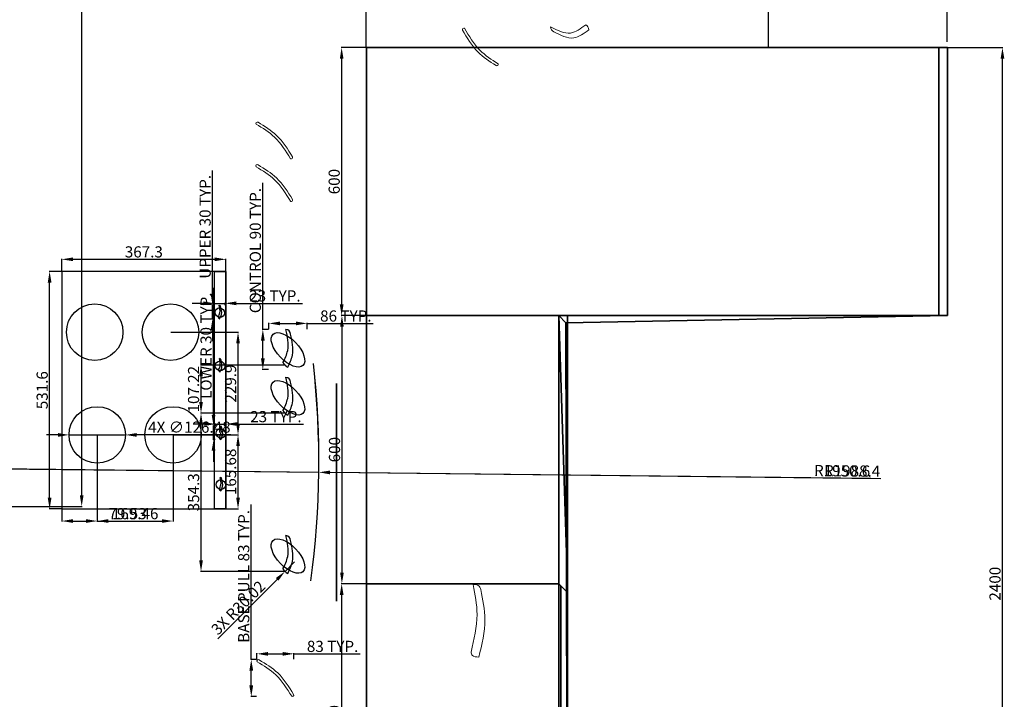
# Model space of a CAD drawing. Units: millimetres. Extents: x 11557 to 15272, y 8572 to 13242.
# Tile 3 of 4: x 13069 to 15272, y 9640 to 11161. Entities that reach past the tile are written whole.
import ezdxf

# ---------------------------------------------------------------- set-up
doc = ezdxf.new("R2010")
doc.units = ezdxf.units.MM
for name, color, linetype, lineweight in [('A-ANNO-DIMS', 2, 'Continuous', 18), ('A-ANNO-REFP', 8, 'Continuous', 13), ('A-EQPM', 9, 'Continuous', 25), ('A-FURN-BASE', 7, 'Continuous', 35), ('A-FURN-HARD', 8, 'Continuous', 18)]:
    doc.layers.add(name, color=color, linetype=linetype, lineweight=lineweight)
doc.styles.get("Standard").update_dxf_attribs({"font": 'arial.ttf'})
doc.dimstyles.new('ISO-25', dxfattribs={"dimtxt": 25, "dimasz": 25, "dimexe": 1.25, "dimexo": 0.625, "dimtad": 1, "dimdec": 1, "dimtxsty": 'Standard', "dimcen": 2.5, "dimadec": 0, "dimazin": 0, "dimtfac": 1, "dimtdec": 1, "dimtmove": 0, "dimatfit": 3, "dimfxl": 1, "dimarcsym": 0})

# ---------------------------------------------------------------- blocks, each defined once
blk = doc.blocks.new('*D2')
at = {"layer": 'A-ANNO-DIMS', "color": 0, "lineweight": -2, "transparency": 16777216}
for p, q in [((13844.6, 9898.9), (13788.4, 9898.9)), ((13789.6, 9873.9), (13789.6, 9323.9)), ((13844.6, 9298.9), (13788.4, 9298.9))]:
    blk.add_line(p, q, dxfattribs=at)
at = {"layer": 'A-ANNO-DIMS', "color": 0, "transparency": 16777216}
for points in [[(13785.5, 9873.9), (13793.8, 9873.9), (13789.6, 9898.9)], [(13785.5, 9323.9), (13793.8, 9323.9), (13789.6, 9298.9)]]:
    blk.add_solid(points, dxfattribs=at)
at = {"layer": 'Defpoints', "color": 0, "transparency": 16777216}
for p in [(13845.2, 9898.9, 720), (13789.6, 9298.9), (13845.2, 9298.9, 720)]:
    blk.add_point(p, dxfattribs=at)
at = {"layer": 'A-ANNO-DIMS', "color": 0, "transparency": 16777216, "insert": (13776.2, 9598.9), "char_height": 25, "attachment_point": 5, "rotation": 90}
blk.add_mtext('600', dxfattribs=at)
blk = doc.blocks.new('*D3')
at = {"layer": 'A-ANNO-DIMS', "color": 0, "lineweight": -2, "transparency": 16777216}
for p, q in [((13845.2, 10498.9), (13789, 10498.9)), ((13790.2, 10473.9), (13790.2, 9923.9)), ((13845.2, 9898.9), (13789, 9898.9))]:
    blk.add_line(p, q, dxfattribs=at)
at = {"layer": 'A-ANNO-DIMS', "color": 0, "transparency": 16777216}
for points in [[(13786.1, 10473.9), (13794.4, 10473.9), (13790.2, 10498.9)], [(13786.1, 9923.9), (13794.4, 9923.9), (13790.2, 9898.9)]]:
    blk.add_solid(points, dxfattribs=at)
at = {"layer": 'Defpoints', "color": 0, "transparency": 16777216}
for p in [(13845.9, 10498.9, 720), (13790.2, 9898.9), (13845.9, 9898.9, 720)]:
    blk.add_point(p, dxfattribs=at)
at = {"layer": 'A-ANNO-DIMS', "color": 0, "transparency": 16777216, "insert": (13776.9, 10198.9), "char_height": 25, "attachment_point": 5, "rotation": 90}
blk.add_mtext('600', dxfattribs=at)
blk = doc.blocks.new('*D4')
at = {"layer": 'A-ANNO-DIMS', "color": 0, "lineweight": -2, "transparency": 16777216}
for p, q in [((13844.6, 11098.9), (13788.4, 11098.9)), ((13789.6, 11073.9), (13789.6, 10523.9)), ((13844.6, 10498.9), (13788.4, 10498.9))]:
    blk.add_line(p, q, dxfattribs=at)
at = {"layer": 'A-ANNO-DIMS', "color": 0, "transparency": 16777216}
for points in [[(13785.5, 11073.9), (13793.8, 11073.9), (13789.6, 11098.9)], [(13785.5, 10523.9), (13793.8, 10523.9), (13789.6, 10498.9)]]:
    blk.add_solid(points, dxfattribs=at)
at = {"layer": 'Defpoints', "color": 0, "transparency": 16777216}
for p in [(13845.2, 11098.9, 720), (13789.6, 10498.9), (13845.2, 10498.9, 720)]:
    blk.add_point(p, dxfattribs=at)
at = {"layer": 'A-ANNO-DIMS', "color": 0, "transparency": 16777216, "insert": (13776.2, 10798.9), "char_height": 25, "attachment_point": 5, "rotation": 90}
blk.add_mtext('600', dxfattribs=at)
blk = doc.blocks.new('*D5')
at = {"layer": 'A-ANNO-DIMS', "color": 0, "lineweight": -2, "transparency": 16777216}
for p, q in [((13844.6, 11098.9), (13844.6, 11236.3)), ((13869.6, 11235), (14719.6, 11235)), ((14744.6, 11098.9), (14744.6, 11236.3))]:
    blk.add_line(p, q, dxfattribs=at)
at = {"layer": 'A-ANNO-DIMS', "color": 0, "transparency": 16777216}
for points in [[(13869.6, 11239.2), (13869.6, 11230.9), (13844.6, 11235)], [(14719.6, 11239.2), (14719.6, 11230.9), (14744.6, 11235)]]:
    blk.add_solid(points, dxfattribs=at)
at = {"layer": 'Defpoints', "color": 0, "transparency": 16777216}
for p in [(14744.6, 11235), (13844.6, 11098.2, 720), (14744.6, 11098.2, 720)]:
    blk.add_point(p, dxfattribs=at)
at = {"layer": 'A-ANNO-DIMS', "color": 0, "transparency": 16777216, "insert": (14294.6, 11248.4), "char_height": 25, "attachment_point": 5}
blk.add_mtext('900', dxfattribs=at)
blk = doc.blocks.new('*D6')
at = {"layer": 'A-ANNO-DIMS', "color": 0, "lineweight": -2, "transparency": 16777216}
for p, q in [((14744.6, 11111.7), (14744.6, 11236.3)), ((15119.6, 11235), (14769.6, 11235)), ((15144.6, 11111.7), (15144.6, 11236.3))]:
    blk.add_line(p, q, dxfattribs=at)
at = {"layer": 'A-ANNO-DIMS', "color": 0, "transparency": 16777216}
for points in [[(14769.6, 11239.2), (14769.6, 11230.9), (14744.6, 11235)], [(15119.6, 11239.2), (15119.6, 11230.9), (15144.6, 11235)]]:
    blk.add_solid(points, dxfattribs=at)
at = {"layer": 'Defpoints', "color": 0, "transparency": 16777216}
for p in [(14744.6, 11235), (14744.6, 11111, 720), (15144.6, 11111, 720)]:
    blk.add_point(p, dxfattribs=at)
at = {"layer": 'A-ANNO-DIMS', "color": 0, "transparency": 16777216, "insert": (14944.6, 11248.4), "char_height": 25, "attachment_point": 5}
blk.add_mtext('400', dxfattribs=at)
blk = doc.blocks.new('BASE-CABINET-PULL')
for centre, radius, start, end in [((3, 79.7, -122.8), 3.04, 50.0455, 215.1607), ((79.2, 3.1, -122.8), 3.13, 238.0113, 27.1949)]:
    blk.add_arc(centre, radius, start, end)
for points in [[(77.6, 0.5, -122.8), (66.9, 17.8, -122.8), (47.2, 49.7, -122.8), (15.2, 69.1, -122.8), (0.5, 77.9, -122.8)], [(82, 4.6, -122.8), (71.3, 21.8, -122.8), (51.6, 53.8, -122.8), (19.6, 73.1, -122.8), (5, 82, -122.8)]]:
    blk.add_open_spline(points, degree=3, knots=[0, 0, 0, 0, 59.935873, 110.632609, 110.632609, 110.632609, 110.632609])
blk = doc.blocks.new('HOB-BURNER')
for centre in [(63.2, 63.2), (63.2, 63.2, -14.7)]:
    blk.add_circle(centre, 63.2)
blk = doc.blocks.new('OVEN-CONTROL')
for centre, radius, start, end in [((31.7, 73), 11.8, 5.8892, 84.1108), ((52.1, 25.8), 30, 210.6614, 239.3386)]:
    blk.add_arc(centre, radius, start, end)
blk.add_ellipse((37.5, 39, 2.5), major_axis=(-33.5, 35), ratio=0.486746)
for points in [[(26.2, 10.5), (30.6, 19.4), (42, 42.9), (36.4, 68.7), (32.9, 84.8)], [(36.8, 0), (41.1, 8.9), (52.5, 32.3), (46.9, 58.2), (43.4, 74.2)]]:
    blk.add_open_spline(points, degree=3, knots=[0, 0, 0, 0, 29.141787, 76.393896, 76.393896, 76.393896, 76.393896])
blk = doc.blocks.new('HOB-CONTROL-LOWER')
for centre, radius, start, end in [((9, 25.8), 4.17, 5.8892, 84.1108), ((16.2, 9.1), 10.6, 210.6614, 239.3386)]:
    blk.add_arc(centre, radius, start, end)
blk.add_ellipse((10.6, 13.6, 1.1), major_axis=(-7.62, 7.96), ratio=0.928231)
for points in [[(7, 3.7), (8.6, 6.9), (12.6, 15.1), (10.6, 24.3), (9.4, 30)], [(10.7, 0), (12.3, 3.2), (16.3, 11.4), (14.3, 20.6), (13.1, 26.2)]]:
    blk.add_open_spline(points, degree=3, knots=[0, 0, 0, 0, 10.30237, 27.007204, 27.007204, 27.007204, 27.007204])
blk = doc.blocks.new('HOB-CONTROL-UPPER')
for centre, radius, start, end in [((9, 25.8, -1.1), 4.17, 5.8892, 84.1108), ((16.2, 9.1, -1.1), 10.6, 210.6614, 239.3386)]:
    blk.add_arc(centre, radius, start, end)
blk.add_ellipse((10.6, 13.6), major_axis=(-7.62, 7.96), ratio=0.928231)
for points in [[(7, 3.7, -1.1), (8.6, 6.9, -1.1), (12.6, 15.1, -1.1), (10.6, 24.3, -1.1), (9.4, 30, -1.1)], [(10.7, 0, -1.1), (12.3, 3.2, -1.1), (16.3, 11.4, -1.1), (14.3, 20.6, -1.1), (13.1, 26.2, -1.1)]]:
    blk.add_open_spline(points, degree=3, knots=[0, 0, 0, 0, 10.30237, 27.007204, 27.007204, 27.007204, 27.007204])
blk = doc.blocks.new('*D21')
at = {"layer": 'A-ANNO-DIMS', "color": 0, "lineweight": -2, "transparency": 16777216}
for p, q in [((13587.4, 9729.4), (13587.4, 10076.2)), ((13599.3, 9729.4), (13586.1, 9729.4)), ((13587.4, 9671.1), (13587.4, 9704.4)), ((13599.3, 9646.1), (13586.1, 9646.1))]:
    blk.add_line(p, q, dxfattribs=at)
at = {"layer": 'A-ANNO-DIMS', "color": 0, "transparency": 16777216}
for points in [[(13583.2, 9704.4), (13591.6, 9704.4), (13587.4, 9729.4)], [(13583.2, 9671.1), (13591.6, 9671.1), (13587.4, 9646.1)]]:
    blk.add_solid(points, dxfattribs=at)
at = {"layer": 'Defpoints', "color": 0, "transparency": 16777216}
for p in [(13587.4, 9729.4), (13599.9, 9729.4), (13599.9, 9646.1)]:
    blk.add_point(p, dxfattribs=at)
at = {"layer": 'A-ANNO-DIMS', "color": 0, "transparency": 16777216, "insert": (13573.8, 9915.3), "char_height": 25, "attachment_point": 5, "rotation": 90}
blk.add_mtext('BASE PULL 83 TYP.', dxfattribs=at)
blk = doc.blocks.new('*D22')
at = {"layer": 'A-ANNO-DIMS', "color": 0, "lineweight": -2, "transparency": 16777216}
for p, q in [((13599.9, 9730), (13599.9, 9743.1)), ((13624.9, 9741.9), (13657.9, 9741.9)), ((13682.9, 9730), (13682.9, 9743.1)), ((13682.9, 9741.9), (13830.8, 9741.9))]:
    blk.add_line(p, q, dxfattribs=at)
at = {"layer": 'A-ANNO-DIMS', "color": 0, "transparency": 16777216}
for points in [[(13624.9, 9746), (13624.9, 9737.7), (13599.9, 9741.9)], [(13657.9, 9746), (13657.9, 9737.7), (13682.9, 9741.9)]]:
    blk.add_solid(points, dxfattribs=at)
at = {"layer": 'Defpoints', "color": 0, "transparency": 16777216}
for p in [(13682.9, 9741.9), (13599.9, 9729.4), (13682.9, 9729.4)]:
    blk.add_point(p, dxfattribs=at)
at = {"layer": 'A-ANNO-DIMS', "color": 0, "transparency": 16777216, "insert": (13769.4, 9755.3), "char_height": 25, "attachment_point": 5}
blk.add_mtext('83 TYP.', dxfattribs=at)
blk = doc.blocks.new('*D23')
at = {"layer": 'A-ANNO-DIMS', "color": 0, "lineweight": -2, "transparency": 16777216}
for p, q in [((13613.3, 10468), (13613.3, 10796.1)), ((13626.1, 10468), (13612, 10468)), ((13613.3, 10403.2), (13613.3, 10443)), ((13626.1, 10378.2), (13612, 10378.2))]:
    blk.add_line(p, q, dxfattribs=at)
at = {"layer": 'A-ANNO-DIMS', "color": 0, "transparency": 16777216}
for points in [[(13609.1, 10443), (13617.5, 10443), (13613.3, 10468)], [(13609.1, 10403.2), (13617.5, 10403.2), (13613.3, 10378.2)]]:
    blk.add_solid(points, dxfattribs=at)
at = {"layer": 'Defpoints', "color": 0, "transparency": 16777216}
for p in [(13613.3, 10468), (13626.8, 10468), (13626.8, 10378.2)]:
    blk.add_point(p, dxfattribs=at)
at = {"layer": 'A-ANNO-DIMS', "color": 0, "transparency": 16777216, "insert": (13599.7, 10644.5), "char_height": 25, "attachment_point": 5, "rotation": 90}
blk.add_mtext('CONTROL 90 TYP.', dxfattribs=at)
blk = doc.blocks.new('*D24')
at = {"layer": 'A-ANNO-DIMS', "color": 0, "lineweight": -2, "transparency": 16777216}
for p, q in [((13626.8, 10468.6), (13626.8, 10482.7)), ((13651.8, 10481.4), (13687.5, 10481.4)), ((13712.5, 10468.6), (13712.5, 10482.7)), ((13712.5, 10481.4), (13860.5, 10481.4))]:
    blk.add_line(p, q, dxfattribs=at)
at = {"layer": 'A-ANNO-DIMS', "color": 0, "transparency": 16777216}
for points in [[(13651.8, 10485.6), (13651.8, 10477.3), (13626.8, 10481.4)], [(13687.5, 10485.6), (13687.5, 10477.3), (13712.5, 10481.4)]]:
    blk.add_solid(points, dxfattribs=at)
at = {"layer": 'Defpoints', "color": 0, "transparency": 16777216}
for p in [(13626.8, 10468), (13712.5, 10481.4), (13712.5, 10468)]:
    blk.add_point(p, dxfattribs=at)
at = {"layer": 'A-ANNO-DIMS', "color": 0, "transparency": 16777216, "insert": (13799, 10494.8), "char_height": 25, "attachment_point": 5}
blk.add_mtext('86 TYP.', dxfattribs=at)
blk = doc.blocks.new('*D29')
at = {"layer": 'A-ANNO-DIMS', "color": 0, "lineweight": -2, "transparency": 16777216}
for p, q in [((13503.1, 10276.7), (13503.1, 10561.3)), ((13506.9, 10251.7), (13501.8, 10251.7)), ((13503.1, 10221.7), (13503.1, 10251.7)), ((13506.9, 10221.7), (13501.8, 10221.7)), ((13503.1, 10196.7), (13503.1, 10171.7))]:
    blk.add_line(p, q, dxfattribs=at)
at = {"layer": 'A-ANNO-DIMS', "color": 0, "transparency": 16777216}
for points in [[(13498.9, 10276.7), (13507.2, 10276.7), (13503.1, 10251.7)], [(13498.9, 10196.7), (13507.2, 10196.7), (13503.1, 10221.7)]]:
    blk.add_solid(points, dxfattribs=at)
at = {"layer": 'Defpoints', "color": 0, "transparency": 16777216}
for p in [(13503.1, 10251.7), (13507.6, 10251.7), (13507.6, 10221.7)]:
    blk.add_point(p, dxfattribs=at)
at = {"layer": 'A-ANNO-DIMS', "color": 0, "transparency": 16777216, "insert": (13489.5, 10431.5), "char_height": 25, "attachment_point": 5, "rotation": 90}
blk.add_mtext('LOWER 30 TYP.', dxfattribs=at)
blk = doc.blocks.new('*D30')
at = {"layer": 'A-ANNO-DIMS', "color": 0, "lineweight": -2, "transparency": 16777216}
for p, q in [((13482.6, 10256.2), (13457.6, 10256.2)), ((13507.6, 10252.3), (13507.6, 10257.4)), ((13507.6, 10256.2), (13531, 10256.2)), ((13531, 10252.3), (13531, 10257.4)), ((13556, 10256.2), (13704.3, 10256.2))]:
    blk.add_line(p, q, dxfattribs=at)
at = {"layer": 'A-ANNO-DIMS', "color": 0, "transparency": 16777216}
for points in [[(13482.6, 10260.4), (13482.6, 10252), (13507.6, 10256.2)], [(13556, 10260.4), (13556, 10252), (13531, 10256.2)]]:
    blk.add_solid(points, dxfattribs=at)
at = {"layer": 'Defpoints', "color": 0, "transparency": 16777216}
for p in [(13507.6, 10251.7), (13531, 10256.2), (13531, 10251.7)]:
    blk.add_point(p, dxfattribs=at)
at = {"layer": 'A-ANNO-DIMS', "color": 0, "transparency": 16777216, "insert": (13642.6, 10269.6), "char_height": 25, "attachment_point": 5}
blk.add_mtext('23 TYP.', dxfattribs=at)
blk = doc.blocks.new('*D31')
at = {"layer": 'A-ANNO-DIMS', "color": 0, "lineweight": -2, "transparency": 16777216}
for p, q in [((13500.8, 10546.9), (13500.8, 10823.6)), ((13504.6, 10521.9), (13499.5, 10521.9)), ((13500.8, 10491.9), (13500.8, 10521.9)), ((13504.6, 10491.9), (13499.5, 10491.9)), ((13500.8, 10466.9), (13500.8, 10441.9))]:
    blk.add_line(p, q, dxfattribs=at)
at = {"layer": 'A-ANNO-DIMS', "color": 0, "transparency": 16777216}
for points in [[(13496.6, 10546.9), (13504.9, 10546.9), (13500.8, 10521.9)], [(13496.6, 10466.9), (13504.9, 10466.9), (13500.8, 10491.9)]]:
    blk.add_solid(points, dxfattribs=at)
at = {"layer": 'Defpoints', "color": 0, "transparency": 16777216}
for p in [(13500.8, 10521.9), (13505.3, 10521.9), (13505.3, 10491.9)]:
    blk.add_point(p, dxfattribs=at)
at = {"layer": 'A-ANNO-DIMS', "color": 0, "transparency": 16777216, "insert": (13487.4, 10697.7), "char_height": 25, "attachment_point": 5, "rotation": 90}
blk.add_mtext('UPPER 30 TYP.', dxfattribs=at)
blk = doc.blocks.new('*D32')
at = {"layer": 'A-ANNO-DIMS', "color": 0, "lineweight": -2, "transparency": 16777216}
for p, q in [((13480.3, 10526.4), (13455.3, 10526.4)), ((13505.3, 10522.5), (13505.3, 10527.6)), ((13505.3, 10526.4), (13528.7, 10526.4)), ((13528.7, 10522.5), (13528.7, 10527.6)), ((13553.7, 10526.4), (13702, 10526.4))]:
    blk.add_line(p, q, dxfattribs=at)
at = {"layer": 'A-ANNO-DIMS', "color": 0, "transparency": 16777216}
for points in [[(13480.3, 10530.6), (13480.3, 10522.2), (13505.3, 10526.4)], [(13553.7, 10530.6), (13553.7, 10522.2), (13528.7, 10526.4)]]:
    blk.add_solid(points, dxfattribs=at)
at = {"layer": 'Defpoints', "color": 0, "transparency": 16777216}
for p in [(13505.3, 10521.9), (13528.7, 10526.4), (13528.7, 10521.9)]:
    blk.add_point(p, dxfattribs=at)
at = {"layer": 'A-ANNO-DIMS', "color": 0, "transparency": 16777216, "insert": (13640.3, 10539.8), "char_height": 25, "attachment_point": 5}
blk.add_mtext('23 TYP.', dxfattribs=at)
blk = doc.blocks.new('*D35')
at = {"layer": 'A-ANNO-DIMS', "color": 0, "lineweight": -2, "transparency": 16777216}
for p, q in [((15145.9, 11098.9), (15269.1, 11098.9)), ((15267.9, 8723.9), (15267.9, 11073.9)), ((14295.9, 8698.9), (15269.1, 8698.9))]:
    blk.add_line(p, q, dxfattribs=at)
at = {"layer": 'A-ANNO-DIMS', "color": 0, "transparency": 16777216}
for points in [[(15263.7, 11073.9), (15272.1, 11073.9), (15267.9, 11098.9)], [(15263.7, 8723.9), (15272.1, 8723.9), (15267.9, 8698.9)]]:
    blk.add_solid(points, dxfattribs=at)
at = {"layer": 'Defpoints', "color": 0, "transparency": 16777216}
for p in [(15145.2, 11098.9), (15267.9, 11098.9), (14295.2, 8698.9)]:
    blk.add_point(p, dxfattribs=at)
at = {"layer": 'A-ANNO-DIMS', "color": 0, "transparency": 16777216, "insert": (15254.5, 9898.9), "char_height": 25, "attachment_point": 5, "rotation": 90}
blk.add_mtext('2400', dxfattribs=at)
blk = doc.blocks.new('*D36')
at = {"layer": 'A-ANNO-DIMS', "color": 0, "lineweight": -2, "transparency": 16777216}
for p, q in [((12944.4, 13071.7), (13209.3, 13071.7)), ((13208.1, 10096.7), (13208.1, 13046.7)), ((11895, 10071.7), (13209.3, 10071.7))]:
    blk.add_line(p, q, dxfattribs=at)
at = {"layer": 'A-ANNO-DIMS', "color": 0, "transparency": 16777216}
for points in [[(13203.9, 13046.7), (13212.2, 13046.7), (13208.1, 13071.7)], [(13203.9, 10096.7), (13212.2, 10096.7), (13208.1, 10071.7)]]:
    blk.add_solid(points, dxfattribs=at)
at = {"layer": 'Defpoints', "color": 0, "transparency": 16777216}
for p in [(12943.8, 13071.7), (13208.1, 13071.7), (11894.4, 10071.7)]:
    blk.add_point(p, dxfattribs=at)
at = {"layer": 'A-ANNO-DIMS', "color": 0, "transparency": 16777216, "insert": (13194.7, 11571.7), "char_height": 25, "attachment_point": 5, "rotation": 90}
blk.add_mtext('3000', dxfattribs=at)
blk = doc.blocks.new('*D41')
at = {"layer": 'A-ANNO-DIMS', "color": 0, "lineweight": -2, "transparency": 16777216}
for p, q in [((13163.4, 10598.5), (13163.4, 10626.2)), ((13188.4, 10624.9), (13505.7, 10624.9)), ((13530.7, 10598.5), (13530.7, 10626.2))]:
    blk.add_line(p, q, dxfattribs=at)
at = {"layer": 'A-ANNO-DIMS', "color": 0, "transparency": 16777216}
for points in [[(13188.4, 10629.1), (13188.4, 10620.8), (13163.4, 10624.9)], [(13505.7, 10629.1), (13505.7, 10620.8), (13530.7, 10624.9)]]:
    blk.add_solid(points, dxfattribs=at)
at = {"layer": 'Defpoints', "color": 0, "transparency": 16777216}
for p in [(13530.7, 10624.9), (13163.4, 10597.8), (13530.7, 10597.8)]:
    blk.add_point(p, dxfattribs=at)
at = {"layer": 'A-ANNO-DIMS', "color": 0, "transparency": 16777216, "insert": (13347.1, 10638.3), "char_height": 25, "attachment_point": 5}
blk.add_mtext('367.3', dxfattribs=at)
blk = doc.blocks.new('*D42')
at = {"layer": 'A-ANNO-DIMS', "color": 0, "lineweight": -2, "transparency": 16777216}
for p, q in [((13162.8, 10597.8), (13135.1, 10597.8)), ((13136.3, 10091.2), (13136.3, 10572.8)), ((13162.8, 10066.2), (13135.1, 10066.2))]:
    blk.add_line(p, q, dxfattribs=at)
at = {"layer": 'A-ANNO-DIMS', "color": 0, "transparency": 16777216}
for points in [[(13132.1, 10572.8), (13140.5, 10572.8), (13136.3, 10597.8)], [(13132.1, 10091.2), (13140.5, 10091.2), (13136.3, 10066.2)]]:
    blk.add_solid(points, dxfattribs=at)
at = {"layer": 'Defpoints', "color": 0, "transparency": 16777216}
for p in [(13136.3, 10597.8), (13163.4, 10597.8), (13163.4, 10066.2)]:
    blk.add_point(p, dxfattribs=at)
at = {"layer": 'A-ANNO-DIMS', "color": 0, "transparency": 16777216, "insert": (13122.9, 10332), "char_height": 25, "attachment_point": 5, "rotation": 90}
blk.add_mtext('531.6', dxfattribs=at)
blk = doc.blocks.new('*D43')
at = {"layer": 'A-ANNO-DIMS', "color": 0, "lineweight": -2, "transparency": 16777216}
for p, q in [((13242.9, 10231.3), (13242.9, 10037.9)), ((13412.4, 10231.3), (13412.4, 10037.9)), ((13267.9, 10039.1), (13387.4, 10039.1))]:
    blk.add_line(p, q, dxfattribs=at)
at = {"layer": 'A-ANNO-DIMS', "color": 0, "transparency": 16777216}
for points in [[(13267.9, 10043.3), (13267.9, 10035), (13242.9, 10039.1)], [(13387.4, 10043.3), (13387.4, 10035), (13412.4, 10039.1)]]:
    blk.add_solid(points, dxfattribs=at)
at = {"layer": 'Defpoints', "color": 0, "transparency": 16777216}
for p in [(13242.9, 10231.9), (13412.4, 10231.9), (13412.4, 10039.1)]:
    blk.add_point(p, dxfattribs=at)
at = {"layer": 'A-ANNO-DIMS', "color": 0, "transparency": 16777216, "insert": (13327.7, 10052.5), "char_height": 25, "attachment_point": 5}
blk.add_mtext('169.46', dxfattribs=at)
blk = doc.blocks.new('*D44')
at = {"layer": 'A-ANNO-DIMS', "color": 0, "lineweight": -2, "transparency": 16777216}
for p, q in [((13407.3, 10461.8), (13559.1, 10461.8)), ((13557.8, 10256.9), (13557.8, 10436.8)), ((13413, 10231.9), (13559.1, 10231.9))]:
    blk.add_line(p, q, dxfattribs=at)
at = {"layer": 'A-ANNO-DIMS', "color": 0, "transparency": 16777216}
for points in [[(13553.7, 10436.8), (13562, 10436.8), (13557.8, 10461.8)], [(13553.7, 10256.9), (13562, 10256.9), (13557.8, 10231.9)]]:
    blk.add_solid(points, dxfattribs=at)
at = {"layer": 'Defpoints', "color": 0, "transparency": 16777216}
for p in [(13406.6, 10461.8), (13557.8, 10461.8), (13412.4, 10231.9)]:
    blk.add_point(p, dxfattribs=at)
at = {"layer": 'A-ANNO-DIMS', "color": 0, "transparency": 16777216, "insert": (13544.4, 10346.8), "char_height": 25, "attachment_point": 5, "rotation": 90}
blk.add_mtext('229.9', dxfattribs=at)
blk = doc.blocks.new('*D45')
at = {"layer": 'A-ANNO-DIMS', "color": 0, "lineweight": -2, "transparency": 16777216}
for p, q in [((13242.9, 10231.3), (13242.9, 10037.9)), ((13163.4, 10065.6), (13163.4, 10037.9)), ((13188.4, 10039.1), (13217.9, 10039.1)), ((13242.9, 10039.1), (13353.4, 10039.1))]:
    blk.add_line(p, q, dxfattribs=at)
at = {"layer": 'A-ANNO-DIMS', "color": 0, "transparency": 16777216}
for points in [[(13188.4, 10043.3), (13188.4, 10035), (13163.4, 10039.1)], [(13217.9, 10043.3), (13217.9, 10035), (13242.9, 10039.1)]]:
    blk.add_solid(points, dxfattribs=at)
at = {"layer": 'Defpoints', "color": 0, "transparency": 16777216}
for p in [(13242.9, 10231.9), (13163.4, 10066.2), (13242.9, 10039.1)]:
    blk.add_point(p, dxfattribs=at)
at = {"layer": 'A-ANNO-DIMS', "color": 0, "transparency": 16777216, "insert": (13310.6, 10052.5), "char_height": 25, "attachment_point": 5}
blk.add_mtext('79.53', dxfattribs=at)
blk = doc.blocks.new('*D46')
at = {"layer": 'A-ANNO-DIMS', "color": 0, "lineweight": -2, "transparency": 16777216}
for p, q in [((13413, 10231.9), (13559.1, 10231.9)), ((13557.8, 10091.2), (13557.8, 10206.9)), ((13531.4, 10066.2), (13559.1, 10066.2))]:
    blk.add_line(p, q, dxfattribs=at)
at = {"layer": 'A-ANNO-DIMS', "color": 0, "transparency": 16777216}
for points in [[(13553.7, 10206.9), (13562, 10206.9), (13557.8, 10231.9)], [(13553.7, 10091.2), (13562, 10091.2), (13557.8, 10066.2)]]:
    blk.add_solid(points, dxfattribs=at)
at = {"layer": 'Defpoints', "color": 0, "transparency": 16777216}
for p in [(13412.4, 10231.9), (13557.8, 10231.9), (13530.7, 10066.2)]:
    blk.add_point(p, dxfattribs=at)
at = {"layer": 'A-ANNO-DIMS', "color": 0, "transparency": 16777216, "insert": (13544.4, 10149.1), "char_height": 25, "attachment_point": 5, "rotation": 90}
blk.add_mtext('165.68', dxfattribs=at)
blk = doc.blocks.new('*D47')
at = {"layer": 'A-ANNO-DIMS', "color": 0, "lineweight": -2, "transparency": 16777216}
for p, q in [((13662.3, 10280.6), (13473.8, 10280.6)), ((13475, 9951.3), (13475, 10255.6)), ((13662.3, 9926.3), (13473.8, 9926.3))]:
    blk.add_line(p, q, dxfattribs=at)
at = {"layer": 'A-ANNO-DIMS', "color": 0, "transparency": 16777216}
for points in [[(13470.8, 10255.6), (13479.2, 10255.6), (13475, 10280.6)], [(13470.8, 9951.3), (13479.2, 9951.3), (13475, 9926.3)]]:
    blk.add_solid(points, dxfattribs=at)
at = {"layer": 'Defpoints', "color": 0, "transparency": 16777216}
for p in [(13475, 10280.6), (13662.9, 10280.6), (13662.9, 9926.3)]:
    blk.add_point(p, dxfattribs=at)
at = {"layer": 'A-ANNO-DIMS', "color": 0, "transparency": 16777216, "insert": (13461.6, 10103.5), "char_height": 25, "attachment_point": 5, "rotation": 90}
blk.add_mtext('354.3', dxfattribs=at)
blk = doc.blocks.new('*D48')
at = {"layer": 'A-ANNO-DIMS', "color": 0, "lineweight": -2, "transparency": 16777216}
for p, q in [((13662.3, 10387.8), (13473.8, 10387.8)), ((13475, 10305.6), (13475, 10362.8)), ((13662.3, 10280.6), (13473.8, 10280.6))]:
    blk.add_line(p, q, dxfattribs=at)
at = {"layer": 'A-ANNO-DIMS', "color": 0, "transparency": 16777216}
for points in [[(13470.8, 10362.8), (13479.2, 10362.8), (13475, 10387.8)], [(13470.8, 10305.6), (13479.2, 10305.6), (13475, 10280.6)]]:
    blk.add_solid(points, dxfattribs=at)
at = {"layer": 'Defpoints', "color": 0, "transparency": 16777216}
for p in [(13475, 10387.8), (13662.9, 10387.8), (13662.9, 10280.6)]:
    blk.add_point(p, dxfattribs=at)
at = {"layer": 'A-ANNO-DIMS', "color": 0, "transparency": 16777216, "insert": (13461.6, 10334.2), "char_height": 25, "attachment_point": 5, "rotation": 90}
blk.add_mtext('107.22', dxfattribs=at)
blk = doc.blocks.new('*D50')
at = {"layer": 'A-ANNO-DIMS', "color": 0, "lineweight": -2, "transparency": 16777216}
for p, q in [((13154.7, 10231.9), (13129.7, 10231.9)), ((13179.7, 10231.9), (13306.2, 10231.9)), ((13541.9, 10231.9), (13331.2, 10231.9))]:
    blk.add_line(p, q, dxfattribs=at)
at = {"layer": 'A-ANNO-DIMS', "color": 0, "transparency": 16777216}
for points in [[(13154.7, 10236.1), (13154.7, 10227.7), (13179.7, 10231.9)], [(13331.2, 10236.1), (13331.2, 10227.7), (13306.2, 10231.9)]]:
    blk.add_solid(points, dxfattribs=at)
at = {"layer": 'Defpoints', "color": 0, "transparency": 16777216}
for p in [(13179.7, 10231.9), (13306.2, 10231.9)]:
    blk.add_point(p, dxfattribs=at)
at = {"layer": 'A-ANNO-DIMS', "color": 0, "transparency": 16777216, "insert": (13449, 10246), "char_height": 25, "attachment_point": 5, "rotation": 359.9999}
blk.add_mtext('4X ∅126.48', dxfattribs=at)
blk = doc.blocks.new('*D51')
at = {"layer": 'A-ANNO-DIMS', "color": 0, "lineweight": -2, "transparency": 16777216}
for p, q in [((13684.2, 9947.5), (13662.9, 9926.3)), ((13512.3, 9775.7), (13645.2, 9908.6))]:
    blk.add_line(p, q, dxfattribs=at)
at = {"layer": 'A-ANNO-DIMS', "color": 0, "transparency": 16777216}
blk.add_solid([(13642.3, 9911.6), (13648.2, 9905.7), (13662.9, 9926.3)], dxfattribs=at)
at = {"layer": 'Defpoints', "color": 0, "transparency": 16777216}
for p in [(13684.2, 9947.5), (13662.9, 9926.3)]:
    blk.add_point(p, dxfattribs=at)
at = {"layer": 'A-ANNO-DIMS', "color": 0, "transparency": 16777216, "insert": (13560.5, 9842.8), "char_height": 25, "attachment_point": 5, "rotation": 45.0002}
blk.add_mtext('3X R30.02', dxfattribs=at)
blk = doc.blocks.new('*D52')
at = {"layer": 'A-ANNO-DIMS', "color": 0, "lineweight": -2, "transparency": 16777216}
for p, q in [((11750.2, 10170.7), (13738.5, 10148.2)), ((14995.9, 10133.9), (13763.5, 10147.9))]:
    blk.add_line(p, q, dxfattribs=at)
at = {"layer": 'A-ANNO-DIMS', "color": 0, "transparency": 16777216}
blk.add_solid([(13763.5, 10152), (13763.4, 10143.7), (13738.5, 10148.2)], dxfattribs=at)
at = {"layer": 'Defpoints', "color": 0, "transparency": 16777216}
for p in [(11750.2, 10170.7), (13738.5, 10148.2)]:
    blk.add_point(p, dxfattribs=at)
at = {"layer": 'A-ANNO-DIMS', "color": 0, "transparency": 16777216, "insert": (14931.6, 10148), "char_height": 25, "attachment_point": 5, "rotation": 359.3508}
blk.add_mtext('R1988.4', dxfattribs=at)
blk = doc.blocks.new('*D53')
at = {"layer": 'A-ANNO-DIMS', "color": 0, "lineweight": -2, "transparency": 16777216}
for p, q in [((11788.3, 10170.3), (13738.8, 10148.2)), ((14973.5, 10134.2), (13763.8, 10147.9))]:
    blk.add_line(p, q, dxfattribs=at)
at = {"layer": 'A-ANNO-DIMS', "color": 0, "transparency": 16777216}
blk.add_solid([(13763.8, 10152), (13763.7, 10143.7), (13738.8, 10148.2)], dxfattribs=at)
at = {"layer": 'Defpoints', "color": 0, "transparency": 16777216}
for p in [(11788.3, 10170.3), (13738.8, 10148.2)]:
    blk.add_point(p, dxfattribs=at)
at = {"layer": 'A-ANNO-DIMS', "color": 0, "transparency": 16777216, "insert": (14909.2, 10148.3), "char_height": 25, "attachment_point": 5, "rotation": 359.3508}
blk.add_mtext('R1950.6', dxfattribs=at)

msp = doc.modelspace()

# ---------------------------------------------------------------- linework, layer by layer
at = {"layer": 'A-ANNO-REFP'}
for p in [(14745.243, 10498.859, 569.986), (14745.243, 10498.859, 419.972), (14745.243, 10498.859, 269.958), (14295.243, 10198.859, 556.518), (14295.243, 10198.859, 393.037), (14295.243, 10198.859, 229.555)]:
    msp.add_point(p, dxfattribs=at)
at = {"layer": 'A-EQPM'}
for p, q in [((13726.305, 10391.552), (13726.305, 10391.552, -30.747)), ((13778.188, 9859.679), (13778.188, 10346.865)), ((13778.188, 10346.865), (13778.188, 10346.865, -218.015)), ((13778.188, 10346.865, -218.015), (13778.188, 9859.679, -218.015)), ((13720.793, 9905.114), (13720.793, 9905.114, -30.747)), ((13778.188, 9859.679, -218.015), (13778.188, 9859.679))]:
    msp.add_line(p, q, dxfattribs=at)
for points in [[(13163.411, 10066.22), (13530.737, 10066.22), (13530.737, 10597.831), (13163.411, 10597.831)], [(13530.737, 10066.22), (13504.841, 10066.22), (13504.841, 10597.831), (13530.737, 10597.831)]]:
    msp.add_lwpolyline(points, close=True, dxfattribs=at)
for centre, radius, start, end in [((11788.258, 10170.261), 1950.639, 352.187696, 6.513961), ((11750.209, 10170.692, -30.747), 1988.4, 352.32442, 6.377237)]:
    msp.add_arc(centre, radius, start, end, dxfattribs=at)
at = {"layer": 'A-FURN-BASE'}
for p, q in [((13845.243, 10498.859, 720), (13845.243, 11098.859, 720)), ((13845.243, 11098.859, 720), (14745.243, 11098.859, 720)), ((14745.243, 11098.859, 720), (15145.243, 11098.859, 720)), ((15125.243, 10498.859, 720), (15125.243, 11098.859, 720)), ((15145.243, 11098.859, 720), (15145.243, 11098.859)), ((15145.243, 10498.859, 720), (15145.243, 11098.859, 720)), ((15145.243, 11098.859), (15145.243, 10498.859)), ((15145.243, 11098.859, 120), (15145.243, 10498.859, 120)), ((15145.243, 11098.859, 140), (15145.243, 10498.859, 140)), ((15145.243, 10528.859, 120), (15145.243, 10528.859)), ((15145.243, 10518.859, 120), (15145.243, 10518.859, 720)), ((15145.243, 10518.859, 120), (15145.243, 10518.859)), ((13845.243, 9898.859, 720), (13845.243, 10498.859, 720)), ((13845.243, 10498.859, 720), (14295.243, 10498.859, 720)), ((13845.243, 10498.859, 720), (14745.243, 10498.859, 720)), ((14275.243, 10498.859, 700), (14295.243, 9898.859, 720)), ((14275.243, 9298.859, 720), (14275.243, 10498.859, 720)), ((14275.243, 10498.859, 720), (14291.462, 10482.64, 136.098)), ((14275.243, 10498.859, 700), (14745.243, 10498.859, 700)), ((15145.243, 10498.859, 120), (14291.462, 10482.64, 136.098)), ((14745.243, 10498.859), (14295.243, 10498.859)), ((14295.243, 10478.859), (14295.243, 10498.859)), ((14295.243, 10498.859), (14295.243, 10498.859, 119.881)), ((14745.243, 10498.859, 720), (15145.243, 10498.859, 720)), ((14745.243, 10498.859, 720), (14745.243, 10498.859, 119.944)), ((14745.243, 10498.859, 569.986), (15145.243, 10498.859, 569.986)), ((14745.243, 10498.859, 419.972), (15145.243, 10498.859, 419.972)), ((14745.243, 10498.859, 269.958), (15145.243, 10498.859, 269.958)), ((15145.243, 10498.859), (14745.243, 10498.859)), ((14745.243, 10498.859, 700), (15145.243, 10498.859, 700)), ((15125.243, 10498.859, 720), (15125.243, 10498.859, 700)), ((15145.243, 10498.859, 120), (15145.243, 10498.859, 720)), ((14291.462, 10482.64, 136.098), (14295.243, 8708.859, 136.098)), ((14295.243, 9278.848), (14295.243, 10478.859)), ((14295.243, 10198.859, 720), (14292.06, 10202.042, 136.098)), ((13845.243, 9298.859, 720), (13845.243, 9898.859, 720)), ((13845.243, 9898.859, 720), (14275.243, 9898.859, 720)), ((14275.243, 9898.859, 720), (14292.744, 9881.358, 136.098)), ((14280.219, 9293.883, 565.291), (14280.219, 9893.883, 565.291)), ((14280.219, 9293.883, 237.922), (14280.219, 9893.883, 237.922)), ((14295.243, 9898.859, 720), (14295.243, 9298.859, 720))]:
    msp.add_line(p, q, dxfattribs=at)
at = {"layer": 'A-FURN-HARD'}
for centre, radius, start, end in [((14330.158, 11138.158), 12.644, 2.326481, 64.265858), ((14330.158, 11138.158, -152.015), 12.644, 2.326481, 64.265858), ((14330.158, 11138.158, -296.009), 12.644, 2.326481, 64.265858), ((14330.158, 11138.158, -441.162), 12.644, 2.326481, 64.265858), ((14062.814, 11139.559), 3.132, 56.524019, 205.70753), ((14269.434, 11145.621), 12.336, 181.465447, 245.126893), ((14269.434, 11145.621, -152.015), 12.336, 181.465447, 245.126893), ((14269.434, 11145.621, -296.009), 12.336, 181.465447, 245.126893), ((14269.434, 11145.621, -441.162), 12.336, 181.465447, 245.126893), ((14136.988, 11061.03), 3.045, 228.55821, 33.673339), ((14087.316, 9883.638), 13.754, 7.963069, 106.22766)]:
    msp.add_arc(centre, radius, start, end, dxfattribs=at)
for points, knots in [([(14257.102, 11145.305), (14272.249, 11137.422), (14299.915, 11123.024), (14324.516, 11141.284), (14335.648, 11149.547)], [0, 0, 0, 0, 46.62950242, 85.16957367, 85.16957367, 85.16957367, 85.16957367]), ([(14257.102, 11145.305, -152.015), (14272.249, 11137.422, -152.015), (14299.915, 11123.024, -152.015), (14324.516, 11141.284, -152.015), (14335.648, 11149.547, -152.015)], [0, 0, 0, 0, 46.62950242, 85.16957367, 85.16957367, 85.16957367, 85.16957367]), ([(14257.102, 11145.305, -296.009), (14272.249, 11137.422, -296.009), (14299.915, 11123.024, -296.009), (14324.516, 11141.284, -296.009), (14335.648, 11149.547, -296.009)], [0, 0, 0, 0, 46.62950242, 85.16957367, 85.16957367, 85.16957367, 85.16957367]), ([(14257.102, 11145.305, -441.162), (14272.249, 11137.422, -441.162), (14299.915, 11123.024, -441.162), (14324.516, 11141.284, -441.162), (14335.648, 11149.547, -441.162)], [0, 0, 0, 0, 46.62950242, 85.16957367, 85.16957367, 85.16957367, 85.16957367]), ([(14059.993, 11138.201), (14070.221, 11120.642), (14089.1, 11088.231), (14120.557, 11068.012), (14134.972, 11058.747)], [0, 0, 0, 0, 59.9358726, 110.63260885, 110.63260885, 110.63260885, 110.63260885]), ([(14064.542, 11142.172), (14074.77, 11124.613), (14093.649, 11092.202), (14125.106, 11071.983), (14139.521, 11062.718)], [0, 0, 0, 0, 59.9358726, 110.63260885, 110.63260885, 110.63260885, 110.63260885]), ([(14264.245, 11134.428), (14279.392, 11126.545), (14307.058, 11112.147), (14331.66, 11130.408), (14342.792, 11138.671)], [0, 0, 0, 0, 46.62950242, 85.16957367, 85.16957367, 85.16957367, 85.16957367]), ([(14264.245, 11134.428, -152.015), (14279.392, 11126.545, -152.015), (14307.058, 11112.147, -152.015), (14331.66, 11130.408, -152.015), (14342.792, 11138.671, -152.015)], [0, 0, 0, 0, 46.62950242, 85.16957367, 85.16957367, 85.16957367, 85.16957367]), ([(14264.245, 11134.428, -296.009), (14279.392, 11126.545, -296.009), (14307.058, 11112.147, -296.009), (14331.66, 11130.408, -296.009), (14342.792, 11138.671, -296.009)], [0, 0, 0, 0, 46.62950242, 85.16957367, 85.16957367, 85.16957367, 85.16957367]), ([(14264.245, 11134.428, -441.162), (14279.392, 11126.545, -441.162), (14307.058, 11112.147, -441.162), (14331.66, 11130.408, -441.162), (14342.792, 11138.671, -441.162)], [0, 0, 0, 0, 46.62950242, 85.16957367, 85.16957367, 85.16957367, 85.16957367]), ([(14079.013, 9745.963), (14085.864, 9773.97), (14098.135, 9824.132), (14087.965, 9874.568), (14083.473, 9896.844)], [0, 0, 0, 0, 85.19241077, 152.5838034, 152.5838034, 152.5838034, 152.5838034]), ([(14096.477, 9734.663), (14103.328, 9762.67), (14115.599, 9812.832), (14105.429, 9863.268), (14100.937, 9885.544)], [0, 0, 0, 0, 85.19241077, 152.5838034, 152.5838034, 152.5838034, 152.5838034]), ([(14079.013, 9745.963), (14079.754, 9743.059), (14081.817, 9734.975), (14090.752, 9734.785), (14096.477, 9734.663)], [0, 0, 0, 0, 8.29929483, 23.09865067, 23.09865067, 23.09865067, 23.09865067])]:
    msp.add_open_spline(points, degree=3, knots=knots, dxfattribs=at)

# ---------------------------------------------------------------- block references
at = {"layer": 'A-EQPM'}
for name, p in [('HOB-BURNER', (13173.941, 10398.555)), ('HOB-BURNER', (13343.404, 10398.555)), ('HOB-CONTROL-UPPER', (13506.349, 10491.943)), ('OVEN-CONTROL', (13632.082, 10383.229)), ('HOB-CONTROL-UPPER', (13506.928, 10372.633)), ('OVEN-CONTROL', (13632.082, 10276.008)), ('HOB-BURNER', (13179.703, 10168.66)), ('HOB-BURNER', (13349.166, 10168.66)), ('HOB-CONTROL-LOWER', (13508.648, 10221.734)), ('HOB-CONTROL-LOWER', (13508.648, 10106.78)), ('OVEN-CONTROL', (13632.082, 9921.718))]:
    msp.add_blockref(name, p, dxfattribs=at)
at = {"layer": 'A-FURN-HARD'}
for p in [(13597.647, 10849.545), (13597.647, 10754.239), (13600.211, 9646.362)]:
    msp.add_blockref('BASE-CABINET-PULL', p, dxfattribs=at)

# ---------------------------------------------------------------- dimensions: what is measured, and where the dimension line sits
at = {"layer": 'A-ANNO-DIMS'}
for base, p1, p2, override, picture, middle in [((13208.076, 13071.656), (11894.396, 10071.656), (12943.771, 13071.656), {"dimdec": 0, "dimlfac": 1, "dimrnd": 0, "dimzin": 0, "dimdsep": 46, "dimlunit": 2}, '*D36', (13194.678, 11571.656)), ((15267.893, 11098.859), (14295.243, 8698.859), (15145.243, 11098.859), {"dimdec": 0, "dimlfac": 1, "dimrnd": 0, "dimzin": 0, "dimdsep": 46, "dimlunit": 2}, '*D35', (15254.503, 9898.859)), ((13136.311, 10597.831), (13163.411, 10066.22), (13163.411, 10597.831), {"dimdec": 1, "dimlfac": 1, "dimrnd": 0, "dimzin": 0, "dimdsep": 46, "dimlunit": 2}, '*D42', (13122.913, 10332.026)), ((13557.837, 10461.797), (13412.407, 10231.902), (13406.646, 10461.797), {"dimdec": 1, "dimlfac": 1, "dimrnd": 0, "dimzin": 0, "dimdsep": 46, "dimlunit": 2}, '*D44', (13544.448, 10346.85)), ((13475.006, 10387.825), (13662.922, 10280.604), (13662.922, 10387.825), {"dimdec": 2, "dimlfac": 1, "dimrnd": 0, "dimzin": 0, "dimdsep": 46, "dimlunit": 2}, '*D48', (13461.617, 10334.214)), ((13475.006, 10280.604), (13662.922, 9926.314), (13662.922, 10280.604), {"dimdec": 1, "dimlfac": 1, "dimrnd": 0, "dimzin": 0, "dimdsep": 46, "dimlunit": 2}, '*D47', (13461.608, 10103.459)), ((13557.837, 10231.902), (13530.737, 10066.22), (13412.407, 10231.902), {"dimdec": 2, "dimlfac": 1, "dimrnd": 0, "dimzin": 0, "dimdsep": 46, "dimlunit": 2}, '*D46', (13544.448, 10149.061))]:
    dim = msp.add_linear_dim(base=base, p1=p1, p2=p2, angle=90, dimstyle='ISO-25', override=override, dxfattribs=at)
    dim.commit()
    dim.dimension.update_dxf_attribs({"geometry": picture, "text_midpoint": middle})
dim = msp.add_linear_dim(base=(14744.618, 11235.018, 720), p1=(13844.618, 11098.234, 1440), p2=(14744.618, 11098.234, 1440), dimstyle='ISO-25', override={"dimclrd": 0, "dimclre": 0, "dimclrt": 0}, dxfattribs=at)
dim.commit()
dim.dimension.update_dxf_attribs({"geometry": '*D5', "text_midpoint": (14294.618, 11235.018, 720), "dimtype": 160})
for base, p1, p2, override, picture, middle in [((14744.618, 11235.018, 720), (15144.618, 11111.04, 1440), (14744.618, 11111.04, 1440), {"dimclrd": 0, "dimclre": 0, "dimclrt": 0}, '*D6', (14944.618, 11248.408, 720)), ((13530.737, 10624.931), (13163.411, 10597.831), (13530.737, 10597.831), {"dimdec": 1, "dimlfac": 1, "dimrnd": 0, "dimzin": 0, "dimdsep": 46, "dimlunit": 2}, '*D41', (13347.074, 10638.329)), ((13242.945, 10039.12), (13163.411, 10066.22), (13242.945, 10231.902), {"dimdec": 2, "dimlfac": 1, "dimrnd": 0, "dimzin": 0, "dimdsep": 46, "dimlunit": 2}, '*D45', (13310.648, 10052.518)), ((13412.407, 10039.12), (13242.945, 10231.902), (13412.407, 10231.902), {"dimdec": 2, "dimlfac": 1, "dimrnd": 0, "dimzin": 0, "dimdsep": 46, "dimlunit": 2}, '*D43', (13327.676, 10052.51))]:
    dim = msp.add_linear_dim(base=base, p1=p1, p2=p2, dimstyle='ISO-25', override=override, dxfattribs=at)
    dim.commit()
    dim.dimension.update_dxf_attribs({"geometry": picture, "text_midpoint": middle})
for base, p1, p2, picture, middle in [((13789.623, 10498.859, 720), (13845.243, 11098.859, 1440), (13845.243, 10498.859, 1440), '*D4', (13789.623, 10798.859, 720)), ((13790.248, 9898.859, 720), (13845.868, 10498.859, 1440), (13845.868, 9898.859, 1440), '*D3', (13790.248, 10198.859, 720)), ((13789.623, 9298.859, 720), (13845.243, 9898.859, 1440), (13845.243, 9298.859, 1440), '*D2', (13789.623, 9598.859, 720))]:
    dim = msp.add_linear_dim(base=base, p1=p1, p2=p2, angle=90, dimstyle='ISO-25', override={"dimclrd": 0, "dimclre": 0, "dimclrt": 0}, dxfattribs=at)
    dim.commit()
    dim.dimension.update_dxf_attribs({"geometry": picture, "text_midpoint": middle, "dimtype": 160})
for base, p1, p2, text, picture, middle in [((13500.768, 10521.906), (13505.263, 10491.943), (13505.263, 10521.906), 'UPPER <> TYP.', '*D31', (13487.37, 10697.744)), ((13613.295, 10467.981), (13626.761, 10378.213), (13626.761, 10467.981), 'CONTROL <> TYP.', '*D23', (13599.735, 10644.536)), ((13503.067, 10251.696), (13507.561, 10221.733), (13507.561, 10251.696), 'LOWER <> TYP.', '*D29', (13489.498, 10431.499)), ((13587.384, 9729.38), (13599.878, 9646.084), (13599.878, 9729.38), 'BASE PULL <> TYP.', '*D21', (13573.824, 9915.271))]:
    dim = msp.add_linear_dim(base=base, p1=p1, p2=p2, angle=90, text=text, dimstyle='ISO-25', override={"dimdec": 0, "dimlfac": 1, "dimrnd": 0, "dimzin": 0, "dimdsep": 46, "dimlunit": 2}, dxfattribs=at)
    dim.commit()
    dim.dimension.update_dxf_attribs({"geometry": picture, "text_midpoint": middle})
for base, p1, p2, picture, middle in [((13528.66, 10526.4), (13505.263, 10521.906), (13528.66, 10521.906), '*D32', (13640.344, 10539.798)), ((13712.497, 10481.446), (13626.761, 10467.981), (13712.497, 10467.981), '*D24', (13798.985, 10494.836)), ((13530.958, 10256.19), (13507.561, 10251.696), (13530.958, 10251.696), '*D30', (13642.642, 10269.588)), ((13682.864, 9741.875), (13599.878, 9729.38), (13682.864, 9729.38), '*D22', (13769.352, 9755.273))]:
    dim = msp.add_linear_dim(base=base, p1=p1, p2=p2, text='<> TYP.', dimstyle='ISO-25', override={"dimdec": 0, "dimlfac": 1, "dimrnd": 0, "dimzin": 0, "dimdsep": 46, "dimlunit": 2}, dxfattribs=at)
    dim.commit()
    dim.dimension.update_dxf_attribs({"geometry": picture, "text_midpoint": middle})
dim = msp.add_diameter_dim_2p(p1=(13179.703, 10231.902), p2=(13306.187, 10231.902), text='4X <>', dimstyle='ISO-25', override={"dimdec": 2, "dimlfac": 1, "dimrnd": 0, "dimzin": 0, "dimdsep": 46, "dimlunit": 2}, dxfattribs=at)
dim.commit()
dim.dimension.update_dxf_attribs({"geometry": '*D50', "text_midpoint": (13449.027, 10231.902)})
for center, mpoint, picture, middle in [((11750.209, 10170.692), (13738.481, 10148.164), '*D52', (14931.444, 10134.647)), ((11788.258, 10170.261), (13738.772, 10148.161), '*D53', (14909.08, 10134.901))]:
    dim = msp.add_radius_dim(center=center, mpoint=mpoint, dimstyle='ISO-25', override={"dimdec": 1, "dimlfac": 1, "dimrnd": 0, "dimzin": 0, "dimdsep": 46, "dimlunit": 2}, dxfattribs=at)
    dim.commit()
    dim.dimension.update_dxf_attribs({"geometry": picture, "text_midpoint": middle, "dimtype": 164})
dim = msp.add_radius_dim(center=(13684.151, 9947.543), mpoint=(13662.922, 9926.314), text='3X <>', dimstyle='ISO-25', override={"dimdec": 2, "dimlfac": 1, "dimrnd": 0, "dimzin": 0, "dimdsep": 46, "dimlunit": 2}, dxfattribs=at)
dim.commit()
dim.dimension.update_dxf_attribs({"geometry": '*D51', "text_midpoint": (13560.47, 9842.809)})

doc.saveas('drawing.dxf')
